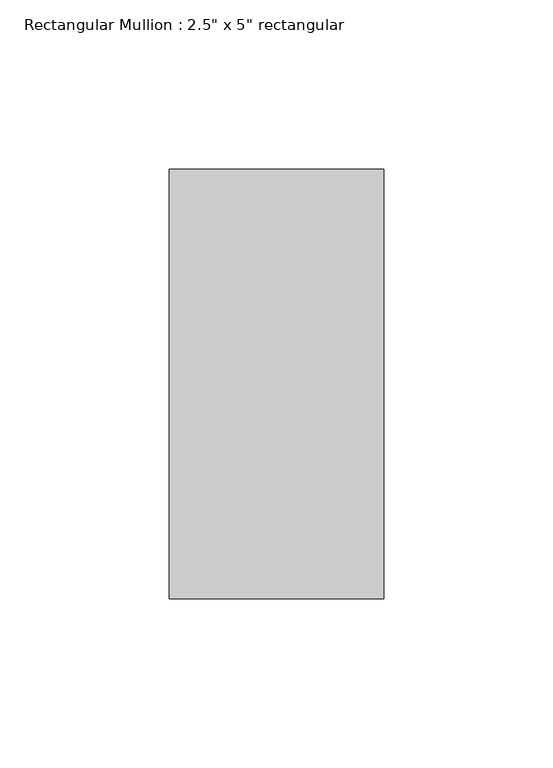
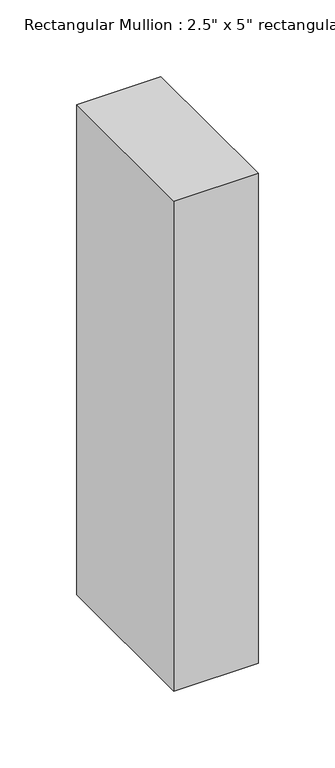
"""IFC4 building model written with IfcOpenShell, lengths in millimetres: member geometry."""

from ifc_helpers import new_model, si_unit, frame, origin, place, context, project, spatial, polyline, outline, extrude, source, transform, mapped, element, save


def member_75a0f14a(model_context):
    return source(origin(), model_context, "Body", "SweptSolid", [
        extrude(outline(polyline([(0.0, 63.5), (0.0, -63.5), (-63.5, -63.5), (-63.5, 63.5), (0.0, 63.5)])), frame((0.0, 0.0, -390.4857245), z_axis=(0.0, 0.0, 1.0), x_axis=(1.0, 0.0, 0.0)), (0.0, 0.0, 1.0), 390.4857245),
    ])


if __name__ == "__main__":
    model = new_model("IFC4")
    model_context = context("Model", 3, world=origin())
    ifc_project = project(units=[si_unit("LENGTHUNIT", "METRE", prefix="MILLI")], contexts=[model_context])
    site = spatial("IfcSite", under=ifc_project)
    building = spatial("IfcBuilding", under=site)
    placement = place(None, origin())
    member_shape = member_75a0f14a(model_context)
    element("IfcMember", 1, ObjectType="Rectangular Mullion : 2.5\" x 5\" rectangular", at=placement, inside=building, context=model_context, shape_type="MappedRepresentation", body=[
        mapped(member_shape, transform((0.0, 0.0, 0.0), x_axis=(1.0, 0.0, 0.0), y_axis=(0.0, 1.0, 0.0), z_axis=(0.0, 0.0, 1.0))),
    ])
    save(model, "model.ifc")

# Revit data of these elements
# Type "Rectangular Mullion : 2.5\" x 5\" rectangular"
#   built-in parameter 1007304 = 0.416667 (stored number, unit not read)
#   built-in parameter 1007301 = 0.104167 (stored number, unit not read)
#   built-in parameter 1007300 = 0.104167 (stored number, unit not read)
# Element 1 (IfcMember, "Rectangular Mullion : 2.5\" x 5\" rectangular")
#   Materials on its faces: "Aluminum"
# Materials
#   "Aluminum": class "Metal", colour RGB 247 247 247, transparency 0, Description = "Aluminum 6061", Cost = 0
